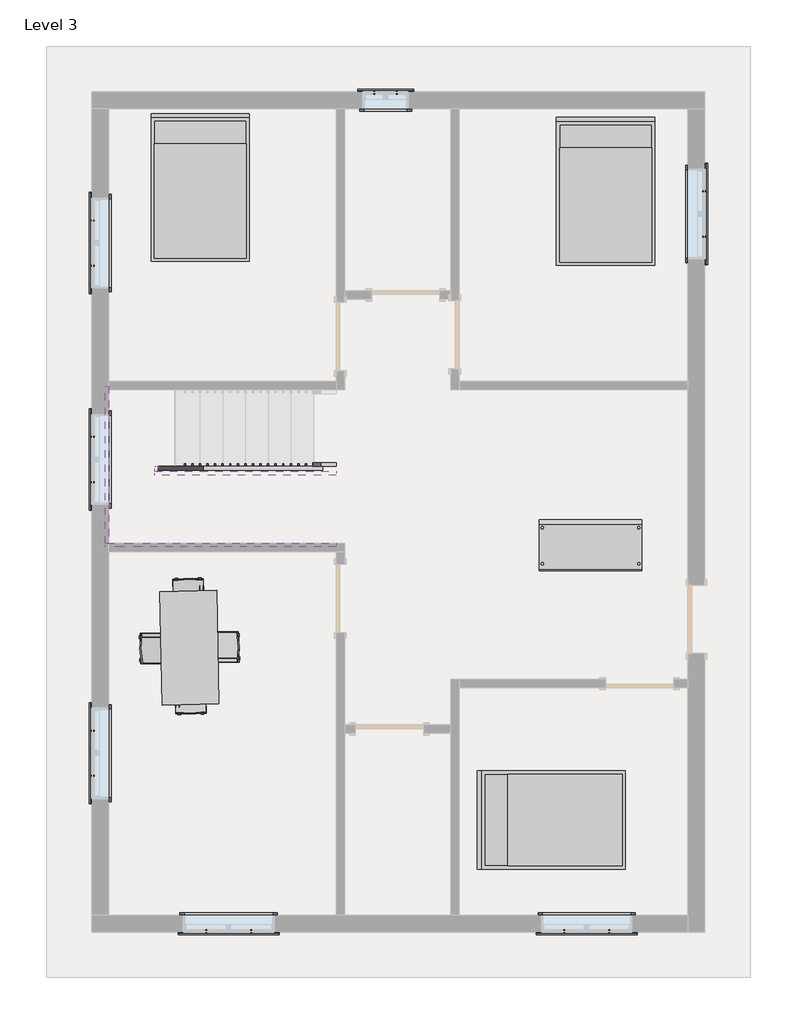
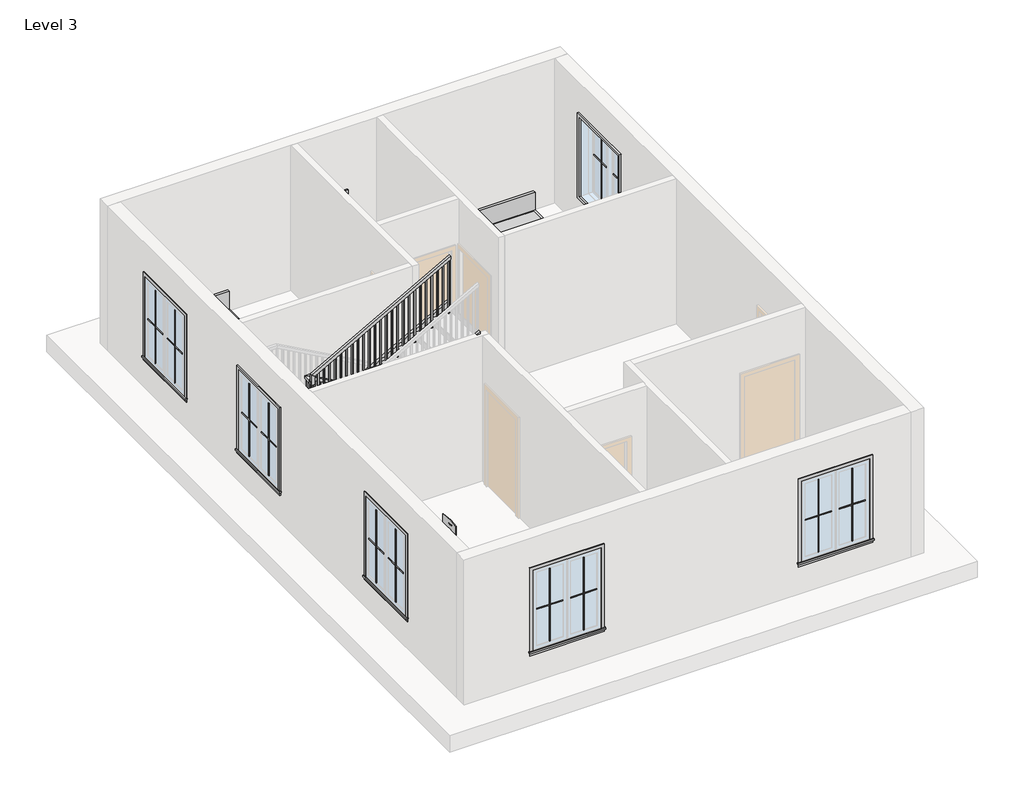
# One storey, part 2 of 2: 29 proxies, 6 members, 4 furniture elements, 1 railing.
"""IFC4 building model written with IfcOpenShell, lengths in millimetres."""

from ifc_helpers import new_model, si_unit, frame, origin, place, context, project, spatial, polyline, outline, extrude, faceted_brep, transform, mapped, element, save
from components import modern_coffee_table_17989_modern_coffee_table_17989_d3a860c8, muntin_pattern_2x2_muntin_pattern_2x2_6dad3731, muntin_pattern_2x2_muntin_pattern_2x2_a30a3345, muntin_pattern_2x2_muntin_pattern_2x2_53152e2c, muntin_pattern_2x2_muntin_pattern_2x2_e8f3e573, trim_window_exterior_flat_with_sill_92b9b949, trim_window_exterior_flat_with_sill_a665a915, trim_window_interior_flat_picture_frame_3bb882cf, trim_window_interior_flat_picture_frame_d485c387, bed_17739_bed_17739_15c61121, dining_table_w_chairs_11374_0cdfc61b

model = new_model("IFC4")

# Units and contexts
model_context = context("Model", 3, world=origin())
ifc_project = project(units=[si_unit("LENGTHUNIT", "METRE", prefix="MILLI")], contexts=[model_context])

# Site, building, storey
site = spatial("IfcSite", under=ifc_project)
building = spatial("IfcBuilding", under=site)
storey = spatial("IfcBuildingStorey", under=building, Name="Level 3", Elevation=6096.0)

# Proxies
placement = place(None, origin())
modern_coffee_table_17989_modern_coffee_table_17989_shape = modern_coffee_table_17989_modern_coffee_table_17989_d3a860c8(model_context)
element("IfcBuildingElementProxy", 1, Name="Modern_Coffee_Table_17989 : Modern_Coffee_Table_17989", ObjectType="Modern_Coffee_Table_17989 : Modern_Coffee_Table_17989", at=placement, inside=storey, context=model_context, shape_type="MappedRepresentation", body=[
    mapped(modern_coffee_table_17989_modern_coffee_table_17989_shape, transform((7937.5, 8234.1992646, 6096.0), x_axis=(1.0, 0.0, 0.0), y_axis=(0.0, 1.0, 0.0), z_axis=(0.0, 0.0, 1.0))),
])
muntin_pattern_2x2_muntin_pattern_2x2_shape = muntin_pattern_2x2_muntin_pattern_2x2_6dad3731(model_context)
element("IfcBuildingElementProxy", 2, Name="Muntin Pattern_2x2 : Muntin Pattern_2x2", ObjectType="Muntin Pattern_2x2 : Muntin Pattern_2x2", at=placement, inside=storey, context=model_context, shape_type="MappedRepresentation", body=[
    mapped(muntin_pattern_2x2_muntin_pattern_2x2_shape, transform((7961.3125, 2701.925, 7080.25), x_axis=(-1.0, 0.0, 0.0), y_axis=(0.0, -1.0, 0.0), z_axis=(0.0, 0.0, 1.0))),
])
element("IfcBuildingElementProxy", 3, Name="Muntin Pattern_2x2 : Muntin Pattern_2x2", ObjectType="Muntin Pattern_2x2 : Muntin Pattern_2x2", at=placement, inside=storey, context=model_context, shape_type="MappedRepresentation", body=[
    mapped(muntin_pattern_2x2_muntin_pattern_2x2_shape, transform((3154.3625, 2701.925, 7080.25), x_axis=(-1.0, 0.0, 0.0), y_axis=(0.0, -1.0, 0.0), z_axis=(0.0, 0.0, 1.0))),
])
element("IfcBuildingElementProxy", 4, Name="Muntin Pattern_2x2 : Muntin Pattern_2x2", ObjectType="Muntin Pattern_2x2 : Muntin Pattern_2x2", at=placement, inside=storey, context=model_context, shape_type="MappedRepresentation", body=[
    mapped(muntin_pattern_2x2_muntin_pattern_2x2_shape, transform((1025.525, 4789.4875, 7080.25), x_axis=(0.0, 1.0, 0.0), y_axis=(-1.0, 0.0, 0.0), z_axis=(0.0, 0.0, 1.0))),
])
element("IfcBuildingElementProxy", 5, Name="Muntin Pattern_2x2 : Muntin Pattern_2x2", ObjectType="Muntin Pattern_2x2 : Muntin Pattern_2x2", at=placement, inside=storey, context=model_context, shape_type="MappedRepresentation", body=[
    mapped(muntin_pattern_2x2_muntin_pattern_2x2_shape, transform((1025.525, 8732.8375, 7080.25), x_axis=(0.0, 1.0, 0.0), y_axis=(-1.0, 0.0, 0.0), z_axis=(0.0, 0.0, 1.0))),
])
element("IfcBuildingElementProxy", 6, Name="Muntin Pattern_2x2 : Muntin Pattern_2x2", ObjectType="Muntin Pattern_2x2 : Muntin Pattern_2x2", at=placement, inside=storey, context=model_context, shape_type="MappedRepresentation", body=[
    mapped(muntin_pattern_2x2_muntin_pattern_2x2_shape, transform((1025.525, 11637.9625, 7080.25), x_axis=(0.0, 1.0, 0.0), y_axis=(-1.0, 0.0, 0.0), z_axis=(0.0, 0.0, 1.0))),
])
element("IfcBuildingElementProxy", 7, Name="Muntin Pattern_2x2 : Muntin Pattern_2x2", ObjectType="Muntin Pattern_2x2 : Muntin Pattern_2x2", at=placement, inside=storey, context=model_context, shape_type="MappedRepresentation", body=[
    mapped(muntin_pattern_2x2_muntin_pattern_2x2_shape, transform((9236.075, 12634.9125, 7080.25), x_axis=(0.0, -1.0, 0.0), y_axis=(1.0, 0.0, 0.0), z_axis=(0.0, 0.0, 1.0))),
])
muntin_pattern_2x2_muntin_pattern_2x2_2_shape = muntin_pattern_2x2_muntin_pattern_2x2_a30a3345(model_context)
element("IfcBuildingElementProxy", 8, Name="Muntin Pattern_2x2 : Muntin Pattern_2x2", ObjectType="Muntin Pattern_2x2 : Muntin Pattern_2x2", at=placement, inside=storey, context=model_context, shape_type="MappedRepresentation", body=[
    mapped(muntin_pattern_2x2_muntin_pattern_2x2_2_shape, transform((7354.8875, 2701.925, 7080.25), x_axis=(1.0, 0.0, 0.0), y_axis=(0.0, 1.0, 0.0), z_axis=(0.0, 0.0, 1.0))),
])
element("IfcBuildingElementProxy", 9, Name="Muntin Pattern_2x2 : Muntin Pattern_2x2", ObjectType="Muntin Pattern_2x2 : Muntin Pattern_2x2", at=placement, inside=storey, context=model_context, shape_type="MappedRepresentation", body=[
    mapped(muntin_pattern_2x2_muntin_pattern_2x2_2_shape, transform((2547.9375, 2701.925, 7080.25), x_axis=(1.0, 0.0, 0.0), y_axis=(0.0, 1.0, 0.0), z_axis=(0.0, 0.0, 1.0))),
])
element("IfcBuildingElementProxy", 10, Name="Muntin Pattern_2x2 : Muntin Pattern_2x2", ObjectType="Muntin Pattern_2x2 : Muntin Pattern_2x2", at=placement, inside=storey, context=model_context, shape_type="MappedRepresentation", body=[
    mapped(muntin_pattern_2x2_muntin_pattern_2x2_2_shape, transform((1025.525, 5395.9125, 7080.25), x_axis=(0.0, -1.0, 0.0), y_axis=(1.0, 0.0, 0.0), z_axis=(0.0, 0.0, 1.0))),
])
element("IfcBuildingElementProxy", 11, Name="Muntin Pattern_2x2 : Muntin Pattern_2x2", ObjectType="Muntin Pattern_2x2 : Muntin Pattern_2x2", at=placement, inside=storey, context=model_context, shape_type="MappedRepresentation", body=[
    mapped(muntin_pattern_2x2_muntin_pattern_2x2_2_shape, transform((1025.525, 9339.2625, 7080.25), x_axis=(0.0, -1.0, 0.0), y_axis=(1.0, 0.0, 0.0), z_axis=(0.0, 0.0, 1.0))),
])
element("IfcBuildingElementProxy", 12, Name="Muntin Pattern_2x2 : Muntin Pattern_2x2", ObjectType="Muntin Pattern_2x2 : Muntin Pattern_2x2", at=placement, inside=storey, context=model_context, shape_type="MappedRepresentation", body=[
    mapped(muntin_pattern_2x2_muntin_pattern_2x2_2_shape, transform((1025.525, 12244.3875, 7080.25), x_axis=(0.0, -1.0, 0.0), y_axis=(1.0, 0.0, 0.0), z_axis=(0.0, 0.0, 1.0))),
])
element("IfcBuildingElementProxy", 13, Name="Muntin Pattern_2x2 : Muntin Pattern_2x2", ObjectType="Muntin Pattern_2x2 : Muntin Pattern_2x2", at=placement, inside=storey, context=model_context, shape_type="MappedRepresentation", body=[
    mapped(muntin_pattern_2x2_muntin_pattern_2x2_2_shape, transform((9236.075, 12028.4875, 7080.25), x_axis=(0.0, 1.0, 0.0), y_axis=(-1.0, 0.0, 0.0), z_axis=(0.0, 0.0, 1.0))),
])
muntin_pattern_2x2_muntin_pattern_2x2_3_shape = muntin_pattern_2x2_muntin_pattern_2x2_53152e2c(model_context)
element("IfcBuildingElementProxy", 14, Name="Muntin Pattern_2x2 : Muntin Pattern_2x2", ObjectType="Muntin Pattern_2x2 : Muntin Pattern_2x2", at=placement, inside=storey, context=model_context, shape_type="MappedRepresentation", body=[
    mapped(muntin_pattern_2x2_muntin_pattern_2x2_3_shape, transform((4808.5375, 13960.475, 7080.25), x_axis=(1.0, 0.0, 0.0), y_axis=(0.0, 1.0, 0.0), z_axis=(0.0, 0.0, 1.0))),
])
muntin_pattern_2x2_muntin_pattern_2x2_4_shape = muntin_pattern_2x2_muntin_pattern_2x2_e8f3e573(model_context)
element("IfcBuildingElementProxy", 15, Name="Muntin Pattern_2x2 : Muntin Pattern_2x2", ObjectType="Muntin Pattern_2x2 : Muntin Pattern_2x2", at=placement, inside=storey, context=model_context, shape_type="MappedRepresentation", body=[
    mapped(muntin_pattern_2x2_muntin_pattern_2x2_4_shape, transform((5110.1625, 13960.475, 7080.25), x_axis=(-1.0, 0.0, 0.0), y_axis=(0.0, -1.0, 0.0), z_axis=(0.0, 0.0, 1.0))),
])
trim_window_exterior_flat_with_sill_shape = trim_window_exterior_flat_with_sill_92b9b949(model_context)
element("IfcBuildingElementProxy", 16, Name="Trim-Window-Exterior-Flat : with Sill", ObjectType="Trim-Window-Exterior-Flat : with Sill", at=placement, inside=storey, context=model_context, shape_type="MappedRepresentation", body=[
    mapped(trim_window_exterior_flat_with_sill_shape, transform((7658.1, 2692.4, 8534.4), x_axis=(1.0, 0.0, 0.0), y_axis=(0.0, 0.0, 1.0), z_axis=(0.0, -1.0, 0.0))),
])
element("IfcBuildingElementProxy", 17, Name="Trim-Window-Exterior-Flat : with Sill", ObjectType="Trim-Window-Exterior-Flat : with Sill", at=placement, inside=storey, context=model_context, shape_type="MappedRepresentation", body=[
    mapped(trim_window_exterior_flat_with_sill_shape, transform((2851.15, 2692.4, 8534.4), x_axis=(1.0, 0.0, 0.0), y_axis=(0.0, 0.0, 1.0), z_axis=(0.0, -1.0, 0.0))),
])
element("IfcBuildingElementProxy", 18, Name="Trim-Window-Exterior-Flat : with Sill", ObjectType="Trim-Window-Exterior-Flat : with Sill", at=placement, inside=storey, context=model_context, shape_type="MappedRepresentation", body=[
    mapped(trim_window_exterior_flat_with_sill_shape, transform((1016.0, 5092.7, 8534.4), x_axis=(0.0, -1.0, 0.0), y_axis=(0.0, 0.0, 1.0), z_axis=(-1.0, 0.0, 0.0))),
])
element("IfcBuildingElementProxy", 19, Name="Trim-Window-Exterior-Flat : with Sill", ObjectType="Trim-Window-Exterior-Flat : with Sill", at=placement, inside=storey, context=model_context, shape_type="MappedRepresentation", body=[
    mapped(trim_window_exterior_flat_with_sill_shape, transform((1016.0, 9036.05, 8534.4), x_axis=(0.0, -1.0, 0.0), y_axis=(0.0, 0.0, 1.0), z_axis=(-1.0, 0.0, 0.0))),
])
element("IfcBuildingElementProxy", 20, Name="Trim-Window-Exterior-Flat : with Sill", ObjectType="Trim-Window-Exterior-Flat : with Sill", at=placement, inside=storey, context=model_context, shape_type="MappedRepresentation", body=[
    mapped(trim_window_exterior_flat_with_sill_shape, transform((1016.0, 11941.175, 8534.4), x_axis=(0.0, -1.0, 0.0), y_axis=(0.0, 0.0, 1.0), z_axis=(-1.0, 0.0, 0.0))),
])
element("IfcBuildingElementProxy", 21, Name="Trim-Window-Exterior-Flat : with Sill", ObjectType="Trim-Window-Exterior-Flat : with Sill", at=placement, inside=storey, context=model_context, shape_type="MappedRepresentation", body=[
    mapped(trim_window_exterior_flat_with_sill_shape, transform((9245.6, 12331.7, 8534.4), x_axis=(0.0, 1.0, 0.0), y_axis=(0.0, 0.0, 1.0), z_axis=(1.0, 0.0, 0.0))),
])
trim_window_exterior_flat_with_sill_2_shape = trim_window_exterior_flat_with_sill_a665a915(model_context)
element("IfcBuildingElementProxy", 22, Name="Trim-Window-Exterior-Flat : with Sill", ObjectType="Trim-Window-Exterior-Flat : with Sill", at=placement, inside=storey, context=model_context, shape_type="MappedRepresentation", body=[
    mapped(trim_window_exterior_flat_with_sill_2_shape, transform((4959.35, 13970.0, 7924.8), x_axis=(-1.0, 0.0, 0.0), y_axis=(0.0, 0.0, 1.0), z_axis=(0.0, 1.0, 0.0))),
])
trim_window_interior_flat_picture_frame_shape = trim_window_interior_flat_picture_frame_3bb882cf(model_context)
element("IfcBuildingElementProxy", 23, Name="Trim-Window-Interior-Flat : Picture Frame", ObjectType="Trim-Window-Interior-Flat : Picture Frame", at=placement, inside=storey, context=model_context, shape_type="MappedRepresentation", body=[
    mapped(trim_window_interior_flat_picture_frame_shape, transform((7658.1, 2921.0, 8534.4), x_axis=(-1.0, 0.0, 0.0), y_axis=(0.0, 0.0, 1.0), z_axis=(0.0, 1.0, 0.0))),
])
element("IfcBuildingElementProxy", 24, Name="Trim-Window-Interior-Flat : Picture Frame", ObjectType="Trim-Window-Interior-Flat : Picture Frame", at=placement, inside=storey, context=model_context, shape_type="MappedRepresentation", body=[
    mapped(trim_window_interior_flat_picture_frame_shape, transform((2851.15, 2921.0, 8534.4), x_axis=(-1.0, 0.0, 0.0), y_axis=(0.0, 0.0, 1.0), z_axis=(0.0, 1.0, 0.0))),
])
element("IfcBuildingElementProxy", 25, Name="Trim-Window-Interior-Flat : Picture Frame", ObjectType="Trim-Window-Interior-Flat : Picture Frame", at=placement, inside=storey, context=model_context, shape_type="MappedRepresentation", body=[
    mapped(trim_window_interior_flat_picture_frame_shape, transform((1244.6, 5092.7, 8534.4), x_axis=(0.0, 1.0, 0.0), y_axis=(0.0, 0.0, 1.0), z_axis=(1.0, 0.0, 0.0))),
])
element("IfcBuildingElementProxy", 26, Name="Trim-Window-Interior-Flat : Picture Frame", ObjectType="Trim-Window-Interior-Flat : Picture Frame", at=placement, inside=storey, context=model_context, shape_type="MappedRepresentation", body=[
    mapped(trim_window_interior_flat_picture_frame_shape, transform((1244.6, 9036.05, 8534.4), x_axis=(0.0, 1.0, 0.0), y_axis=(0.0, 0.0, 1.0), z_axis=(1.0, 0.0, 0.0))),
])
element("IfcBuildingElementProxy", 27, Name="Trim-Window-Interior-Flat : Picture Frame", ObjectType="Trim-Window-Interior-Flat : Picture Frame", at=placement, inside=storey, context=model_context, shape_type="MappedRepresentation", body=[
    mapped(trim_window_interior_flat_picture_frame_shape, transform((1244.6, 11941.175, 8534.4), x_axis=(0.0, 1.0, 0.0), y_axis=(0.0, 0.0, 1.0), z_axis=(1.0, 0.0, 0.0))),
])
element("IfcBuildingElementProxy", 28, Name="Trim-Window-Interior-Flat : Picture Frame", ObjectType="Trim-Window-Interior-Flat : Picture Frame", at=placement, inside=storey, context=model_context, shape_type="MappedRepresentation", body=[
    mapped(trim_window_interior_flat_picture_frame_shape, transform((9017.0, 12331.7, 8534.4), x_axis=(0.0, -1.0, 0.0), y_axis=(0.0, 0.0, 1.0), z_axis=(-1.0, 0.0, 0.0))),
])
trim_window_interior_flat_picture_frame_2_shape = trim_window_interior_flat_picture_frame_d485c387(model_context)
element("IfcBuildingElementProxy", 29, Name="Trim-Window-Interior-Flat : Picture Frame", ObjectType="Trim-Window-Interior-Flat : Picture Frame", at=placement, inside=storey, context=model_context, shape_type="MappedRepresentation", body=[
    mapped(trim_window_interior_flat_picture_frame_2_shape, transform((4959.35, 13741.4, 7924.8), x_axis=(1.0, 0.0, 0.0), y_axis=(0.0, 0.0, 1.0), z_axis=(0.0, -1.0, 0.0))),
])

# Furniture
bed_17739_bed_17739_shape = bed_17739_bed_17739_15c61121(model_context)
element("IfcFurniture", 30, ObjectType="Bed_17739 : Bed_17739", at=placement, inside=storey, context=model_context, shape_type="MappedRepresentation", body=[
    mapped(bed_17739_bed_17739_shape, transform((2470.15, 12661.9, 6096.0), x_axis=(1.0, 0.0, 0.0), y_axis=(0.0, 1.0, 0.0), z_axis=(0.0, 0.0, 1.0))),
])
element("IfcFurniture", 31, ObjectType="Bed_17739 : Bed_17739", at=placement, inside=storey, context=model_context, shape_type="MappedRepresentation", body=[
    mapped(bed_17739_bed_17739_shape, transform((7912.1, 12611.1, 6096.0), x_axis=(1.0, 0.0, 0.0), y_axis=(0.0, 1.0, 0.0), z_axis=(0.0, 0.0, 1.0))),
])
element("IfcFurniture", 32, ObjectType="Bed_17739 : Bed_17739", at=placement, inside=storey, context=model_context, shape_type="MappedRepresentation", body=[
    mapped(bed_17739_bed_17739_shape, transform((7207.25, 4197.35, 6096.0), x_axis=(0.0, 1.0, 0.0), y_axis=(-1.0, 0.0, 0.0), z_axis=(0.0, 0.0, 1.0))),
])
dining_table_w_chairs_11374_shape = dining_table_w_chairs_11374_0cdfc61b(model_context)
element("IfcFurniture", 33, ObjectType="Dining_Table_w_Chairs_11374", at=placement, inside=storey, context=model_context, shape_type="MappedRepresentation", body=[
    mapped(dining_table_w_chairs_11374_shape, transform((2420.6366388, 6492.5326572, 6096.0), x_axis=(-0.019560245774115807, 0.9998086800909743, 0.0), y_axis=(-0.9998086800909743, -0.019560245774115807, 0.0), z_axis=(0.0, 0.0, 1.0))),
])

# Members
element("IfcMember", 34, ObjectType="Stringer - 2\" Width", at=placement, inside=storey, context=model_context, shape_type="SweptSolid", body=[
    extrude(outline(polyline([(6096.0, 4295.1355783), (6303.5983948, 4295.1355783), (7630.0428392, 1907.5355783), (7281.3641651, 1907.5355783), (6096.0, 4041.1910755), (6096.0, 4295.1355783)])), frame((0.0, 8893.8068332, 0.0), z_axis=(0.0, 1.0, 0.0), x_axis=(0.0, 0.0, 1.0)), (0.0, 0.0, 1.0), 50.8),
])
element("IfcMember", 35, ObjectType="Stringer - 2\" Width", at=placement, inside=storey, context=model_context, shape_type="SweptSolid", body=[
    extrude(outline(polyline([(1856.7355783, 8944.6068332), (1907.5355783, 8944.6068332), (1907.5355783, 8877.3), (1856.7355783, 8877.3), (1856.7355783, 8944.6068332)])), frame((0.0, 0.0, 7391.4), z_axis=(0.0, 0.0, 1.0), x_axis=(1.0, 0.0, 0.0)), (0.0, 0.0, 1.0), 304.8),
])
element("IfcMember", 36, ObjectType="Stringer - 2\" Width", at=placement, inside=storey, context=model_context, shape_type="SweptSolid", body=[
    extrude(outline(polyline([(7827.5983948, 1856.7355783), (7478.9197207, 1856.7355783), (8833.5863873, 4295.1355783), (9182.2650614, 4295.1355783), (7827.5983948, 1856.7355783)])), frame((0.0, 8826.5, 0.0), z_axis=(0.0, 1.0, 0.0), x_axis=(0.0, 0.0, 1.0)), (0.0, 0.0, 1.0), 50.8),
])
element("IfcMember", 37, ObjectType="Stringer - 2\" Width", at=placement, inside=storey, context=model_context, shape_type="SweptSolid", body=[
    extrude(outline(polyline([(6096.0, 4295.1355783), (6303.5983948, 4295.1355783), (7696.2, 1788.4526889), (7696.2, 1244.6), (7649.6617086, 1244.6), (6096.0, 4041.1910755), (6096.0, 4295.1355783)])), frame((0.0, 9969.5, 0.0), z_axis=(0.0, 1.0, 0.0), x_axis=(0.0, 0.0, 1.0)), (0.0, 0.0, 1.0), 50.8),
])
element("IfcMember", 38, ObjectType="Stringer - 2\" Width", at=placement, inside=storey, context=model_context, shape_type="SweptSolid", body=[
    extrude(outline(polyline([(1193.8, 10020.3), (1244.6, 10020.3), (1244.6, 7912.1), (1193.8, 7912.1), (1193.8, 10020.3)])), frame((0.0, 0.0, 7391.4), z_axis=(0.0, 0.0, 1.0), x_axis=(1.0, 0.0, 0.0)), (0.0, 0.0, 1.0), 304.8),
])
element("IfcMember", 39, ObjectType="Stringer - 2\" Width", at=placement, inside=storey, context=model_context, shape_type="SweptSolid", body=[
    extrude(outline(polyline([(7459.3008513, 1193.8), (7391.4, 1193.8), (7391.4, 1699.2000811), (8833.5863873, 4295.1355783), (9182.2650614, 4295.1355783), (7459.3008513, 1193.8)])), frame((0.0, 7861.3, 0.0), z_axis=(0.0, 1.0, 0.0), x_axis=(0.0, 0.0, 1.0)), (0.0, 0.0, 1.0), 50.8),
])

# Railing
element("IfcRailing", 40, ObjectType="Handrail - Rectangular", at=placement, inside=storey, context=model_context, shape_type="SolidModel", body=[
    faceted_brep([(4295.1355783, 8944.6068332, 7179.7333333), (4295.1355783, 8944.6068332, 7121.620221), (4295.1355783, 8995.4068332, 7121.620221), (4295.1355783, 8995.4068332, 7179.7333333), (1932.9355783, 8944.6068332, 8492.0666667), (1882.1355783, 8944.6068332, 8462.1757765), (1882.1355783, 8995.4068332, 8462.1757765), (1932.9355783, 8995.4068332, 8492.0666667), (1932.9355783, 8944.6068332, 8534.4), (1882.1355783, 8944.6068332, 8483.6), (1882.1355783, 8995.4068332, 8483.6), (1932.9355783, 8995.4068332, 8534.4), (1856.7355783, 8944.6068332, 8534.4), (1856.7355783, 8944.6068332, 8483.6), (1805.9355783, 8995.4068332, 8483.6), (1805.9355783, 8995.4068332, 8534.4), (1856.7355783, 8868.4068332, 8534.4), (1856.7355783, 8868.4068332, 8483.6), (1805.9355783, 8868.4068332, 8483.6), (1805.9355783, 8868.4068332, 8534.4), (1856.7355783, 8826.5, 8534.4), (1805.9355783, 8826.5, 8534.4), (1805.9355783, 8775.7, 8483.6), (1856.7355783, 8775.7, 8483.6)], [[[0, 1, 2, 3]], [[1, 0, 4, 5]], [[2, 1, 5, 6]], [[3, 2, 6, 7]], [[0, 3, 7, 4]], [[5, 4, 8, 9]], [[6, 5, 9, 10]], [[7, 6, 10, 11]], [[4, 7, 11, 8]], [[9, 8, 12, 13]], [[10, 9, 13, 14]], [[11, 10, 14, 15]], [[8, 11, 15, 12]], [[13, 12, 16, 17]], [[14, 13, 17, 18]], [[15, 14, 18, 19]], [[12, 15, 19, 16]], [[20, 21, 22, 23]], [[17, 16, 20, 23]], [[18, 17, 23, 22]], [[19, 18, 22, 21]], [[16, 19, 21, 20]]]),
    faceted_brep([(1856.7355783, 8826.5, 8534.4), (1856.7355783, 8775.7, 8483.6), (1805.9355783, 8775.7, 8483.6), (1805.9355783, 8826.5, 8534.4), (1856.7355783, 8826.5, 8645.620221), (1805.9355783, 8826.5, 8675.5111111), (1805.9355783, 8775.7, 8675.5111111), (1856.7355783, 8775.7, 8645.620221)], [[[0, 1, 2, 3]], [[4, 5, 6, 7]], [[1, 0, 4, 7]], [[2, 1, 7, 6]], [[3, 2, 6, 5]], [[0, 3, 5, 4]]]),
    faceted_brep([(1805.9355783, 8826.5, 8675.5111111), (1856.7355783, 8826.5, 8645.620221), (1856.7355783, 8775.7, 8645.620221), (1805.9355783, 8775.7, 8675.5111111), (4295.1355783, 8826.5, 10058.4), (4295.1355783, 8775.7, 10058.4), (4295.1355783, 8775.7, 10000.2868876), (4295.1355783, 8826.5, 10000.2868876)], [[[0, 1, 2, 3]], [[4, 5, 6, 7]], [[1, 0, 4, 7]], [[2, 1, 7, 6]], [[3, 2, 6, 5]], [[0, 3, 5, 4]]]),
    extrude(outline(polyline([(9980.8841099, 4260.2105783), (8974.6666667, 4260.2105783), (8974.6666667, 4279.2605783), (9991.4674432, 4279.2605783), (9980.8841099, 4260.2105783)])), frame((0.0, 8791.575, 0.0), z_axis=(0.0, 1.0, 0.0), x_axis=(0.0, 0.0, 1.0)), (0.0, 0.0, 1.0), 19.05),
    extrude(outline(polyline([(9924.4396654, 4158.6105783), (8974.6666667, 4158.6105783), (8974.6666667, 4177.6605783), (9935.0229988, 4177.6605783), (9924.4396654, 4158.6105783)])), frame((0.0, 8791.575, 0.0), z_axis=(0.0, 1.0, 0.0), x_axis=(0.0, 0.0, 1.0)), (0.0, 0.0, 1.0), 19.05),
    extrude(outline(polyline([(9867.995221, 4057.0105783), (8974.6666667, 4057.0105783), (8974.6666667, 4076.0605783), (9878.5785543, 4076.0605783), (9867.995221, 4057.0105783)])), frame((0.0, 8791.575, 0.0), z_axis=(0.0, 1.0, 0.0), x_axis=(0.0, 0.0, 1.0)), (0.0, 0.0, 1.0), 19.05),
    extrude(outline(polyline([(9811.5507765, 3955.4105783), (8805.3333333, 3955.4105783), (8805.3333333, 3974.4605783), (9822.1341099, 3974.4605783), (9811.5507765, 3955.4105783)])), frame((0.0, 8791.575, 0.0), z_axis=(0.0, 1.0, 0.0), x_axis=(0.0, 0.0, 1.0)), (0.0, 0.0, 1.0), 19.05),
    extrude(outline(polyline([(9755.1063321, 3853.8105783), (8805.3333333, 3853.8105783), (8805.3333333, 3872.8605783), (9765.6896654, 3872.8605783), (9755.1063321, 3853.8105783)])), frame((0.0, 8791.575, 0.0), z_axis=(0.0, 1.0, 0.0), x_axis=(0.0, 0.0, 1.0)), (0.0, 0.0, 1.0), 19.05),
    extrude(outline(polyline([(9698.6618876, 3752.2105783), (8805.3333333, 3752.2105783), (8805.3333333, 3771.2605783), (9709.245221, 3771.2605783), (9698.6618876, 3752.2105783)])), frame((0.0, 8791.575, 0.0), z_axis=(0.0, 1.0, 0.0), x_axis=(0.0, 0.0, 1.0)), (0.0, 0.0, 1.0), 19.05),
    extrude(outline(polyline([(9642.2174432, 3650.6105783), (8636.0, 3650.6105783), (8636.0, 3669.6605783), (9652.8007765, 3669.6605783), (9642.2174432, 3650.6105783)])), frame((0.0, 8791.575, 0.0), z_axis=(0.0, 1.0, 0.0), x_axis=(0.0, 0.0, 1.0)), (0.0, 0.0, 1.0), 19.05),
    extrude(outline(polyline([(9585.7729988, 3549.0105783), (8636.0, 3549.0105783), (8636.0, 3568.0605783), (9596.3563321, 3568.0605783), (9585.7729988, 3549.0105783)])), frame((0.0, 8791.575, 0.0), z_axis=(0.0, 1.0, 0.0), x_axis=(0.0, 0.0, 1.0)), (0.0, 0.0, 1.0), 19.05),
    extrude(outline(polyline([(9529.3285543, 3447.4105783), (8636.0, 3447.4105783), (8636.0, 3466.4605783), (9539.9118876, 3466.4605783), (9529.3285543, 3447.4105783)])), frame((0.0, 8791.575, 0.0), z_axis=(0.0, 1.0, 0.0), x_axis=(0.0, 0.0, 1.0)), (0.0, 0.0, 1.0), 19.05),
    extrude(outline(polyline([(9472.8841099, 3345.8105783), (8466.6666667, 3345.8105783), (8466.6666667, 3364.8605783), (9483.4674432, 3364.8605783), (9472.8841099, 3345.8105783)])), frame((0.0, 8791.575, 0.0), z_axis=(0.0, 1.0, 0.0), x_axis=(0.0, 0.0, 1.0)), (0.0, 0.0, 1.0), 19.05),
    extrude(outline(polyline([(9416.4396654, 3244.2105783), (8466.6666667, 3244.2105783), (8466.6666667, 3263.2605783), (9427.0229988, 3263.2605783), (9416.4396654, 3244.2105783)])), frame((0.0, 8791.575, 0.0), z_axis=(0.0, 1.0, 0.0), x_axis=(0.0, 0.0, 1.0)), (0.0, 0.0, 1.0), 19.05),
    extrude(outline(polyline([(9359.995221, 3142.6105783), (8466.6666667, 3142.6105783), (8466.6666667, 3161.6605783), (9370.5785543, 3161.6605783), (9359.995221, 3142.6105783)])), frame((0.0, 8791.575, 0.0), z_axis=(0.0, 1.0, 0.0), x_axis=(0.0, 0.0, 1.0)), (0.0, 0.0, 1.0), 19.05),
    extrude(outline(polyline([(9303.5507765, 3041.0105783), (8297.3333333, 3041.0105783), (8297.3333333, 3060.0605783), (9314.1341099, 3060.0605783), (9303.5507765, 3041.0105783)])), frame((0.0, 8791.575, 0.0), z_axis=(0.0, 1.0, 0.0), x_axis=(0.0, 0.0, 1.0)), (0.0, 0.0, 1.0), 19.05),
    extrude(outline(polyline([(9247.1063321, 2939.4105783), (8297.3333333, 2939.4105783), (8297.3333333, 2958.4605783), (9257.6896654, 2958.4605783), (9247.1063321, 2939.4105783)])), frame((0.0, 8791.575, 0.0), z_axis=(0.0, 1.0, 0.0), x_axis=(0.0, 0.0, 1.0)), (0.0, 0.0, 1.0), 19.05),
    extrude(outline(polyline([(9190.6618876, 2837.8105783), (8297.3333333, 2837.8105783), (8297.3333333, 2856.8605783), (9201.245221, 2856.8605783), (9190.6618876, 2837.8105783)])), frame((0.0, 8791.575, 0.0), z_axis=(0.0, 1.0, 0.0), x_axis=(0.0, 0.0, 1.0)), (0.0, 0.0, 1.0), 19.05),
    extrude(outline(polyline([(9134.2174432, 2736.2105783), (8128.0, 2736.2105783), (8128.0, 2755.2605783), (9144.8007765, 2755.2605783), (9134.2174432, 2736.2105783)])), frame((0.0, 8791.575, 0.0), z_axis=(0.0, 1.0, 0.0), x_axis=(0.0, 0.0, 1.0)), (0.0, 0.0, 1.0), 19.05),
    extrude(outline(polyline([(9077.7729988, 2634.6105783), (8128.0, 2634.6105783), (8128.0, 2653.6605783), (9088.3563321, 2653.6605783), (9077.7729988, 2634.6105783)])), frame((0.0, 8791.575, 0.0), z_axis=(0.0, 1.0, 0.0), x_axis=(0.0, 0.0, 1.0)), (0.0, 0.0, 1.0), 19.05),
    extrude(outline(polyline([(9021.3285543, 2533.0105783), (8128.0, 2533.0105783), (8128.0, 2552.0605783), (9031.9118876, 2552.0605783), (9021.3285543, 2533.0105783)])), frame((0.0, 8791.575, 0.0), z_axis=(0.0, 1.0, 0.0), x_axis=(0.0, 0.0, 1.0)), (0.0, 0.0, 1.0), 19.05),
    extrude(outline(polyline([(8964.8841099, 2431.4105783), (7958.6666667, 2431.4105783), (7958.6666667, 2450.4605783), (8975.4674432, 2450.4605783), (8964.8841099, 2431.4105783)])), frame((0.0, 8791.575, 0.0), z_axis=(0.0, 1.0, 0.0), x_axis=(0.0, 0.0, 1.0)), (0.0, 0.0, 1.0), 19.05),
    extrude(outline(polyline([(8908.4396654, 2329.8105783), (7958.6666667, 2329.8105783), (7958.6666667, 2348.8605783), (8919.0229988, 2348.8605783), (8908.4396654, 2329.8105783)])), frame((0.0, 8791.575, 0.0), z_axis=(0.0, 1.0, 0.0), x_axis=(0.0, 0.0, 1.0)), (0.0, 0.0, 1.0), 19.05),
    extrude(outline(polyline([(8851.995221, 2228.2105783), (7958.6666667, 2228.2105783), (7958.6666667, 2247.2605783), (8862.5785543, 2247.2605783), (8851.995221, 2228.2105783)])), frame((0.0, 8791.575, 0.0), z_axis=(0.0, 1.0, 0.0), x_axis=(0.0, 0.0, 1.0)), (0.0, 0.0, 1.0), 19.05),
    extrude(outline(polyline([(8795.5507765, 2126.6105783), (7789.3333333, 2126.6105783), (7789.3333333, 2145.6605783), (8806.1341099, 2145.6605783), (8795.5507765, 2126.6105783)])), frame((0.0, 8791.575, 0.0), z_axis=(0.0, 1.0, 0.0), x_axis=(0.0, 0.0, 1.0)), (0.0, 0.0, 1.0), 19.05),
    extrude(outline(polyline([(8739.1063321, 2025.0105783), (7789.3333333, 2025.0105783), (7789.3333333, 2044.0605783), (8749.6896654, 2044.0605783), (8739.1063321, 2025.0105783)])), frame((0.0, 8791.575, 0.0), z_axis=(0.0, 1.0, 0.0), x_axis=(0.0, 0.0, 1.0)), (0.0, 0.0, 1.0), 19.05),
    extrude(outline(polyline([(8682.6618876, 1923.4105783), (7789.3333333, 1923.4105783), (7789.3333333, 1942.4605783), (8693.245221, 1942.4605783), (8682.6618876, 1923.4105783)])), frame((0.0, 8791.575, 0.0), z_axis=(0.0, 1.0, 0.0), x_axis=(0.0, 0.0, 1.0)), (0.0, 0.0, 1.0), 19.05),
    extrude(outline(polyline([(1840.8605783, 8877.9318332), (1840.8605783, 8858.8818332), (1821.8105783, 8858.8818332), (1821.8105783, 8877.9318332), (1840.8605783, 8877.9318332)])), frame((0.0, 0.0, 7620.0), z_axis=(0.0, 0.0, 1.0), x_axis=(1.0, 0.0, 0.0)), (0.0, 0.0, 1.0), 863.6),
    extrude(outline(polyline([(1866.2605783, 8960.4818332), (1847.2105783, 8960.4818332), (1847.2105783, 8979.5318332), (1866.2605783, 8979.5318332), (1866.2605783, 8960.4818332)])), frame((0.0, 0.0, 7620.0), z_axis=(0.0, 0.0, 1.0), x_axis=(1.0, 0.0, 0.0)), (0.0, 0.0, 1.0), 863.6),
    extrude(outline(polyline([(8425.1341099, 1948.8105783), (7450.6666667, 1948.8105783), (7450.6666667, 1967.8605783), (8414.5507765, 1967.8605783), (8425.1341099, 1948.8105783)])), frame((0.0, 8960.4818332, 0.0), z_axis=(0.0, 1.0, 0.0), x_axis=(0.0, 0.0, 1.0)), (0.0, 0.0, 1.0), 19.05),
    extrude(outline(polyline([(8368.6896654, 2050.4105783), (7450.6666667, 2050.4105783), (7450.6666667, 2069.4605783), (8358.1063321, 2069.4605783), (8368.6896654, 2050.4105783)])), frame((0.0, 8960.4818332, 0.0), z_axis=(0.0, 1.0, 0.0), x_axis=(0.0, 0.0, 1.0)), (0.0, 0.0, 1.0), 19.05),
    extrude(outline(polyline([(8312.245221, 2152.0105783), (7450.6666667, 2152.0105783), (7450.6666667, 2171.0605783), (8301.6618876, 2171.0605783), (8312.245221, 2152.0105783)])), frame((0.0, 8960.4818332, 0.0), z_axis=(0.0, 1.0, 0.0), x_axis=(0.0, 0.0, 1.0)), (0.0, 0.0, 1.0), 19.05),
    extrude(outline(polyline([(8255.8007765, 2253.6105783), (7281.3333333, 2253.6105783), (7281.3333333, 2272.6605783), (8245.2174432, 2272.6605783), (8255.8007765, 2253.6105783)])), frame((0.0, 8960.4818332, 0.0), z_axis=(0.0, 1.0, 0.0), x_axis=(0.0, 0.0, 1.0)), (0.0, 0.0, 1.0), 19.05),
    extrude(outline(polyline([(8199.3563321, 2355.2105783), (7281.3333333, 2355.2105783), (7281.3333333, 2374.2605783), (8188.7729988, 2374.2605783), (8199.3563321, 2355.2105783)])), frame((0.0, 8960.4818332, 0.0), z_axis=(0.0, 1.0, 0.0), x_axis=(0.0, 0.0, 1.0)), (0.0, 0.0, 1.0), 19.05),
    extrude(outline(polyline([(8142.9118876, 2456.8105783), (7281.3333333, 2456.8105783), (7281.3333333, 2475.8605783), (8132.3285543, 2475.8605783), (8142.9118876, 2456.8105783)])), frame((0.0, 8960.4818332, 0.0), z_axis=(0.0, 1.0, 0.0), x_axis=(0.0, 0.0, 1.0)), (0.0, 0.0, 1.0), 19.05),
    extrude(outline(polyline([(8086.4674432, 2558.4105783), (7112.0, 2558.4105783), (7112.0, 2577.4605783), (8075.8841099, 2577.4605783), (8086.4674432, 2558.4105783)])), frame((0.0, 8960.4818332, 0.0), z_axis=(0.0, 1.0, 0.0), x_axis=(0.0, 0.0, 1.0)), (0.0, 0.0, 1.0), 19.05),
    extrude(outline(polyline([(8030.0229988, 2660.0105783), (7112.0, 2660.0105783), (7112.0, 2679.0605783), (8019.4396654, 2679.0605783), (8030.0229988, 2660.0105783)])), frame((0.0, 8960.4818332, 0.0), z_axis=(0.0, 1.0, 0.0), x_axis=(0.0, 0.0, 1.0)), (0.0, 0.0, 1.0), 19.05),
    extrude(outline(polyline([(7973.5785543, 2761.6105783), (7112.0, 2761.6105783), (7112.0, 2780.6605783), (7962.995221, 2780.6605783), (7973.5785543, 2761.6105783)])), frame((0.0, 8960.4818332, 0.0), z_axis=(0.0, 1.0, 0.0), x_axis=(0.0, 0.0, 1.0)), (0.0, 0.0, 1.0), 19.05),
    extrude(outline(polyline([(7917.1341099, 2863.2105783), (6942.6666667, 2863.2105783), (6942.6666667, 2882.2605783), (7906.5507765, 2882.2605783), (7917.1341099, 2863.2105783)])), frame((0.0, 8960.4818332, 0.0), z_axis=(0.0, 1.0, 0.0), x_axis=(0.0, 0.0, 1.0)), (0.0, 0.0, 1.0), 19.05),
    extrude(outline(polyline([(7860.6896654, 2964.8105783), (6942.6666667, 2964.8105783), (6942.6666667, 2983.8605783), (7850.1063321, 2983.8605783), (7860.6896654, 2964.8105783)])), frame((0.0, 8960.4818332, 0.0), z_axis=(0.0, 1.0, 0.0), x_axis=(0.0, 0.0, 1.0)), (0.0, 0.0, 1.0), 19.05),
    extrude(outline(polyline([(7804.245221, 3066.4105783), (6942.6666667, 3066.4105783), (6942.6666667, 3085.4605783), (7793.6618876, 3085.4605783), (7804.245221, 3066.4105783)])), frame((0.0, 8960.4818332, 0.0), z_axis=(0.0, 1.0, 0.0), x_axis=(0.0, 0.0, 1.0)), (0.0, 0.0, 1.0), 19.05),
    extrude(outline(polyline([(7747.8007765, 3168.0105783), (6773.3333333, 3168.0105783), (6773.3333333, 3187.0605783), (7737.2174432, 3187.0605783), (7747.8007765, 3168.0105783)])), frame((0.0, 8960.4818332, 0.0), z_axis=(0.0, 1.0, 0.0), x_axis=(0.0, 0.0, 1.0)), (0.0, 0.0, 1.0), 19.05),
    extrude(outline(polyline([(7691.3563321, 3269.6105783), (6773.3333333, 3269.6105783), (6773.3333333, 3288.6605783), (7680.7729988, 3288.6605783), (7691.3563321, 3269.6105783)])), frame((0.0, 8960.4818332, 0.0), z_axis=(0.0, 1.0, 0.0), x_axis=(0.0, 0.0, 1.0)), (0.0, 0.0, 1.0), 19.05),
    extrude(outline(polyline([(7634.9118876, 3371.2105783), (6773.3333333, 3371.2105783), (6773.3333333, 3390.2605783), (7624.3285543, 3390.2605783), (7634.9118876, 3371.2105783)])), frame((0.0, 8960.4818332, 0.0), z_axis=(0.0, 1.0, 0.0), x_axis=(0.0, 0.0, 1.0)), (0.0, 0.0, 1.0), 19.05),
    extrude(outline(polyline([(7578.4674432, 3472.8105783), (6604.0, 3472.8105783), (6604.0, 3491.8605783), (7567.8841099, 3491.8605783), (7578.4674432, 3472.8105783)])), frame((0.0, 8960.4818332, 0.0), z_axis=(0.0, 1.0, 0.0), x_axis=(0.0, 0.0, 1.0)), (0.0, 0.0, 1.0), 19.05),
    extrude(outline(polyline([(7522.0229988, 3574.4105783), (6604.0, 3574.4105783), (6604.0, 3593.4605783), (7511.4396654, 3593.4605783), (7522.0229988, 3574.4105783)])), frame((0.0, 8960.4818332, 0.0), z_axis=(0.0, 1.0, 0.0), x_axis=(0.0, 0.0, 1.0)), (0.0, 0.0, 1.0), 19.05),
    extrude(outline(polyline([(7465.5785543, 3676.0105783), (6604.0, 3676.0105783), (6604.0, 3695.0605783), (7454.995221, 3695.0605783), (7465.5785543, 3676.0105783)])), frame((0.0, 8960.4818332, 0.0), z_axis=(0.0, 1.0, 0.0), x_axis=(0.0, 0.0, 1.0)), (0.0, 0.0, 1.0), 19.05),
    extrude(outline(polyline([(7409.1341099, 3777.6105783), (6434.6666667, 3777.6105783), (6434.6666667, 3796.6605783), (7398.5507765, 3796.6605783), (7409.1341099, 3777.6105783)])), frame((0.0, 8960.4818332, 0.0), z_axis=(0.0, 1.0, 0.0), x_axis=(0.0, 0.0, 1.0)), (0.0, 0.0, 1.0), 19.05),
    extrude(outline(polyline([(7352.6896654, 3879.2105783), (6434.6666667, 3879.2105783), (6434.6666667, 3898.2605783), (7342.1063321, 3898.2605783), (7352.6896654, 3879.2105783)])), frame((0.0, 8960.4818332, 0.0), z_axis=(0.0, 1.0, 0.0), x_axis=(0.0, 0.0, 1.0)), (0.0, 0.0, 1.0), 19.05),
    extrude(outline(polyline([(7296.245221, 3980.8105783), (6434.6666667, 3980.8105783), (6434.6666667, 3999.8605783), (7285.6618876, 3999.8605783), (7296.245221, 3980.8105783)])), frame((0.0, 8960.4818332, 0.0), z_axis=(0.0, 1.0, 0.0), x_axis=(0.0, 0.0, 1.0)), (0.0, 0.0, 1.0), 19.05),
    extrude(outline(polyline([(7239.8007765, 4082.4105783), (6265.3333333, 4082.4105783), (6265.3333333, 4101.4605783), (7229.2174432, 4101.4605783), (7239.8007765, 4082.4105783)])), frame((0.0, 8960.4818332, 0.0), z_axis=(0.0, 1.0, 0.0), x_axis=(0.0, 0.0, 1.0)), (0.0, 0.0, 1.0), 19.05),
    extrude(outline(polyline([(7183.3563321, 4184.0105783), (6265.3333333, 4184.0105783), (6265.3333333, 4203.0605783), (7172.7729988, 4203.0605783), (7183.3563321, 4184.0105783)])), frame((0.0, 8960.4818332, 0.0), z_axis=(0.0, 1.0, 0.0), x_axis=(0.0, 0.0, 1.0)), (0.0, 0.0, 1.0), 19.05),
    extrude(outline(polyline([(1840.8605783, 8810.625), (1840.8605783, 8791.575), (1821.8105783, 8791.575), (1821.8105783, 8810.625), (1840.8605783, 8810.625)])), frame((0.0, 0.0, 7620.0), z_axis=(0.0, 0.0, 1.0), x_axis=(1.0, 0.0, 0.0)), (0.0, 0.0, 1.0), 863.6),
    extrude(outline(polyline([(1840.8605783, 8960.4818332), (1821.8105783, 8960.4818332), (1821.8105783, 8979.5318332), (1840.8605783, 8979.5318332), (1840.8605783, 8960.4818332)])), frame((0.0, 0.0, 7620.0), z_axis=(0.0, 0.0, 1.0), x_axis=(1.0, 0.0, 0.0)), (0.0, 0.0, 1.0), 863.6),
    extrude(outline(polyline([(9989.7035543, 4276.0855783), (8974.6666667, 4276.0855783), (8974.6666667, 4295.1355783), (10000.2868876, 4295.1355783), (9989.7035543, 4276.0855783)])), frame((0.0, 8791.575, 0.0), z_axis=(0.0, 1.0, 0.0), x_axis=(0.0, 0.0, 1.0)), (0.0, 0.0, 1.0), 19.05),
    extrude(outline(polyline([(7132.2035543, 4276.0855783), (6265.3333333, 4276.0855783), (6265.3333333, 4295.1355783), (7121.620221, 4295.1355783), (7132.2035543, 4276.0855783)])), frame((0.0, 8960.4818332, 0.0), z_axis=(0.0, 1.0, 0.0), x_axis=(0.0, 0.0, 1.0)), (0.0, 0.0, 1.0), 19.05),
])

save(model, "model.ifc")

# Revit data of these elements
# Type "Modern_Coffee_Table_17989 : Modern_Coffee_Table_17989"
#   Default Elevation = 0
# Type "Muntin Pattern_2x2 : Muntin Pattern_2x2"
#   Width [instance default] = 4' - 0"
#   Thickness = 0' - 0 1/2"
#   Height [instance default] = 4' - 0"
#   Distance = 0' - 0 3/4"
#   Interior Material [instance default] = none
#   Exterior Material [instance default] = none
#   Default Elevation = 0
# Type "Trim-Window-Exterior-Flat : with Sill"
#   Trim Width = 0' - 2 1/4"
#   Trim Thickness_Picture Frame = 0' - 1 1/4"
#   Trim Thickness_with Sill = 0' - 0 3/4"
#   Sill Thickness = 0' - 1 1/4"
#   Opening Width [instance default] = 2' - 0"
#   Opening Height [instance default] = 3' - 0"
#   Default Elevation = 4' - 0"
#   Sill = yes
#   Picture Frame = no
#   Trim Material [instance default] = none
# Type "Trim-Window-Interior-Flat : Picture Frame"
#   Trim Thickness_Picture Frame = 0' - 1 1/4"
#   Trim Width = 0' - 2 1/4"
#   Trim Thickness_with Sill = 0' - 0 3/4"
#   Sill Thickness = 0' - 1 1/4"
#   Opening Width [instance default] = 2' - 0"
#   Opening Height [instance default] = 3' - 0"
#   Default Elevation = 4' - 0"
#   Sill = no
#   Picture Frame = yes
#   Trim Material [instance default] = none
# Type "Bed_17739 : Bed_17739"
#   Default Elevation = 0
# Type "Dining_Table_w_Chairs_11374"
#   Default Elevation = 0
#   Assembly Code = ""
# Type "Handrail - Rectangular"
#   Assembly Code = "C2010400"
#   built-in parameter 1008612 = 0.0416667 (stored number, unit not read)
#   built-in parameter 1008611 = 0.0416667 (stored number, unit not read)
#   built-in parameter 1008609 = 0.333333 (stored number, unit not read)
#   built-in parameter 1008604 = 0.166667 (stored number, unit not read)
#   built-in parameter 1008603 = 0.166667 (stored number, unit not read)
#   Railing Height = 3' - 0"
#   built-in parameter 1008630 = 2
#   built-in parameter 1008610 = 2
#   built-in parameter 1008618 = Baluster - Square : 3/4"
# Element 1 (IfcBuildingElementProxy, "Modern_Coffee_Table_17989 : Modern_Coffee_Table_17989")
#   Phase Created = New Construction
#   Materials on its faces: "1 Wood", "1 Glass", "1 Metal"
# Elements 2, 3, 4, 5, 6, 7, 8, 9, 10, 11, 12, 13 (IfcBuildingElementProxy, "Muntin Pattern_2x2 : Muntin Pattern_2x2")
#   Width = 1' - 6 5/8"
#   Height = 4' - 6 1/2"
#   Interior Material = Wood - Stained
#   Exterior Material = Clad - White
#   Phase Created = New Construction
#   Materials on its faces: "Clad - White", "Wood - Stained"
# Elements 14, 15 (IfcBuildingElementProxy, "Muntin Pattern_2x2 : Muntin Pattern_2x2")
#   Width = 0' - 6 5/8"
#   Height = 2' - 6 1/2"
#   Interior Material = Wood - Stained
#   Exterior Material = Clad - White
#   Phase Created = New Construction
#   Materials on its faces: "Clad - White", "Wood - Stained"
# Elements 16, 17, 18, 19, 20, 21 (IfcBuildingElementProxy, "Trim-Window-Exterior-Flat : with Sill")
#   Opening Width = 4' - 0"
#   Opening Height = 5' - 0"
#   Trim Material = Clad - White
#   Phase Created = New Construction
#   Materials on its faces: "Clad - White"
# Element 22 (IfcBuildingElementProxy, "Trim-Window-Exterior-Flat : with Sill")
#   Opening Width = 2' - 0"
#   Opening Height = 3' - 0"
#   Trim Material = Clad - White
#   Phase Created = New Construction
#   Materials on its faces: "Clad - White"
# Elements 23, 24, 25, 26, 27, 28 (IfcBuildingElementProxy, "Trim-Window-Interior-Flat : Picture Frame")
#   Opening Width = 4' - 0"
#   Opening Height = 5' - 0"
#   Trim Material = Wood - Stained
#   Phase Created = New Construction
#   Materials on its faces: "Wood - Stained"
# Element 29 (IfcBuildingElementProxy, "Trim-Window-Interior-Flat : Picture Frame")
#   Opening Width = 2' - 0"
#   Opening Height = 3' - 0"
#   Trim Material = Wood - Stained
#   Phase Created = New Construction
#   Materials on its faces: "Wood - Stained"
# Elements 30, 31, 32 (IfcFurniture, "Bed_17739 : Bed_17739")
#   Phase Created = New Construction
#   Materials on its faces: "legs", "sheets", "bed frame", "Blanket"
# Element 33 (IfcFurniture, "Dining_Table_w_Chairs_11374")
#   Phase Created = New Construction
# Elements 34, 35, 36, 37, 38, 39 (IfcMember, "Stringer - 2\" Width")
#   Phase Created = New Construction
# Element 40 (IfcRailing, "Handrail - Rectangular")
#   Phase Created = New Construction
# Materials
#   "1 Wood": class "Glass", colour RGB 81 52 39, transparency 0, Cost = 0
#   "1 Glass": class "Glass", colour RGB 236 240 239, transparency 0.85, Cost = 0
#   "1 Metal": class "Glass", colour RGB 244 244 244, transparency 0, Cost = 0
#   "Clad - White": class "Wood", colour RGB 242 242 238, transparency 0, Cost = 0
#   "Wood - Stained": class "Wood", colour RGB 224 178 126, transparency 0, Cost = 0
#   "legs": colour RGB 90 73 37, transparency 0, Cost = 0
#   "sheets": colour RGB 200 195 176, transparency 0, Cost = 0
#   "bed frame": colour RGB 90 73 37, transparency 0, Cost = 0
#   "Blanket": class "System", colour RGB 59 0 1, transparency 0, Cost = 0
